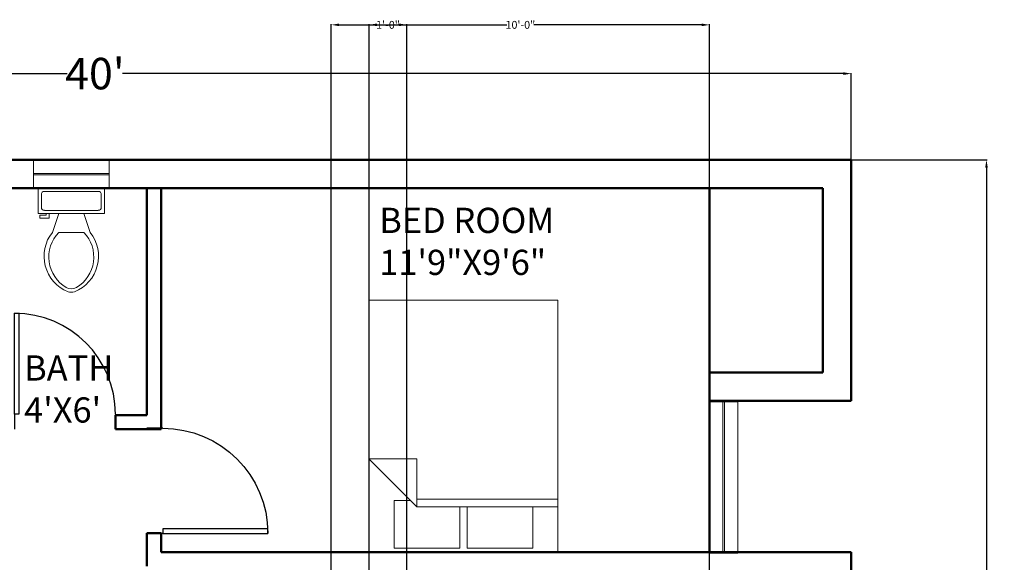
# Model space of a CAD drawing. Units: inches. Extents: x -46 to 565, y -56 to 809.
# Tile 6 of 6: x 252 to 565, y 636 to 809. Entities that reach past the tile are written whole.
import ezdxf

# ---------------------------------------------------------------- set-up
doc = ezdxf.new("R2010")
doc.units = ezdxf.units.IN
doc.header["$MEASUREMENT"] = 0
for name, color, linetype, lineweight in [('A-ANNO-DIMS', 2, 'Continuous', 18), ('A-AREA-IDEN', 241, 'Continuous', 18), ('A-FLOR-FIXT', 131, 'Continuous', 18), ('A-FURN', 131, 'Continuous', 18), ('DOOR', 210, 'Continuous', 25), ('WALL', 10, 'Continuous', 50), ('WINDOW', 170, 'Continuous', 18)]:
    doc.layers.add(name, color=color, linetype=linetype, lineweight=lineweight)
doc.styles.get("Standard").update_dxf_attribs({"font": 'arial.ttf'})
doc.dimstyles.get("Standard").update_dxf_attribs({"dimtxt": 2.5, "dimasz": 2.5, "dimexe": 0.18, "dimexo": 0.0625, "dimgap": 0.09, "dimtad": 0, "dimtih": 1, "dimtoh": 1, "dimzin": 0, "dimdsep": 46, "dimlunit": 3, "dimtxsty": 'Standard', "dimcen": 0.09, "dimadec": 0, "dimazin": 0, "dimtfac": 1, "dimtofl": 0, "dimtmove": 0, "dimatfit": 3, "dimfxl": 1, "dimtolj": 1, "dimtzin": 0, "dimarcsym": 0})

# ---------------------------------------------------------------- blocks, each defined once
blk = doc.blocks.new('*U2')
for p, q in [((0, 0), (0, -6)), ((40, 0), (40, -6))]:
    blk.add_line(p, q)
blk.add_lwpolyline([(0, 0), (0, 40), (1.75, 40), (1.75, 0)], close=True)
blk.add_arc((0, 0), 40, 0, 90)
blk = doc.blocks.new('Bed - Queen')
for p, q in [((0, -80.00003), (0, 0)), ((0, 0), (59.99999, 0)), ((59.99999, 0), (59.99999, -80.00003)), ((7.99999, -1.2), (28.79998, -1.2)), ((7.99999, -14.4), (7.99999, -1.2)), ((28.79998, -1.2), (28.79998, -14.4)), ((31.19999, -1.2), (51.99999, -1.2)), ((31.19999, -14.4), (31.19999, -1.2)), ((51.99999, -1.2), (51.99999, -16.4)), ((0, -14.4), (44.8, -14.4)), ((59.99999, -29.6), (44.8, -14.4)), ((44.8, -14.4), (44.8, -29.6)), ((44.8, -16.8), (0, -16.8)), ((51.99999, -16.4), (46.79936, -16.4)), ((44.8, -29.6), (59.99999, -29.6)), ((59.99999, -80.00003), (0, -80.00003))]:
    blk.add_line(p, q)
blk = doc.blocks.new('Toilet - top')
for p, q in [((9.5, -6), (9.5, -2)), ((-10, -8.5), (-8, -8.5)), ((-10, -9.5), (-10, -8.5)), ((-8, -8.5), (-8, -8)), ((-7, -8), (-7, -9.5)), ((-4, -8), (-6, -14)), ((4, -8), (6, -14)), ((-7, -9.5), (-10, -9.5)), ((4, -14), (-4, -14))]:
    blk.add_line(p, q)
blk.add_lwpolyline([(10.5, -8), (10.5, 0), (-10.5, 0), (-10.5, -8)], close=True)
for points in [[(-9.5, -2), (-9.5, -6)], [(8.5, -1), (-8.5, -1)], [(-8.5, -7), (8.5, -7)]]:
    blk.add_lwpolyline(points)
for centre, radius, start, end in [((-8.62, -1.88), 0.884, 81.8699, 188.1301), ((8.62, -1.88), 0.884, 351.8699, 98.1301), ((-8.62, -6.12), 0.884, 171.8699, 278.1301), ((8.62, -6.12), 0.884, 261.8699, 8.1301), ((3.52, -21.58), 12.17, 141.4691, 247.9714), ((4.2, -21.82), 11.33, 136.3677, 238.9468), ((-3.52, -21.58), 12.17, 292.0284, 38.5307), ((-4.2, -21.82), 11.33, 301.053, 43.6321), ((0, -27.88), 4, 245.7318, 294.2682), ((0, -29), 4, 254.8605, 285.1395)]:
    blk.add_arc(centre, radius, start, end)
blk = doc.blocks.new('*D14')
at = {"layer": 'A-ANNO-DIMS', "color": 0, "lineweight": -2, "transparency": 16777216}
for p, q in [((36.14, 764.26), (36.14, 791.8)), ((38.64, 791.62), (267.37, 791.62)), ((513.64, 791.62), (284.92, 791.62)), ((516.14, 764.26), (516.14, 791.8))]:
    blk.add_line(p, q, dxfattribs=at)
at = {"layer": 'A-ANNO-DIMS', "color": 0, "transparency": 16777216}
for points in [[(38.64, 792.04), (38.64, 791.2), (36.14, 791.62)], [(513.64, 792.04), (513.64, 791.2), (516.14, 791.62)]]:
    blk.add_solid(points, dxfattribs=at)
at = {"layer": 'Defpoints', "color": 0, "transparency": 16777216}
for p in [(516.14, 791.62), (36.14, 764.2), (516.14, 764.2)]:
    blk.add_point(p, dxfattribs=at)
at = {"layer": 'A-ANNO-DIMS', "color": 0, "transparency": 16777216, "insert": (276.14, 791.62), "char_height": 10, "attachment_point": 5}
blk.add_mtext("\\A1;40'", dxfattribs=at)
blk = doc.blocks.new('WIN-48IN')
for p, q in [((0, 4.75), (48, 4.75)), ((0, 4.25), (48, 4.25))]:
    blk.add_line(p, q)
blk.add_lwpolyline([(0, 0), (48, 0), (48, 9), (0, 9)], close=True)
blk = doc.blocks.new('WIN-24IN')
for p, q in [((4.25, 24), (4.25, 0)), ((4.75, 24), (4.75, 0))]:
    blk.add_line(p, q)
blk.add_lwpolyline([(0, 24), (0, 0), (9, 0), (9, 24)], close=True)
blk = doc.blocks.new('*D39')
at = {"layer": 'A-ANNO-DIMS', "color": 0, "lineweight": -2, "transparency": 16777216}
for p, q in [((516.21, 764.2), (559.22, 764.2)), ((559.04, 761.7), (559.04, 610.07)), ((559.04, 455.7), (559.04, 607.33)), ((507.21, 453.2), (559.22, 453.2))]:
    blk.add_line(p, q, dxfattribs=at)
at = {"layer": 'A-ANNO-DIMS', "color": 0, "transparency": 16777216}
for points in [[(558.63, 761.7), (559.46, 761.7), (559.04, 764.2)], [(558.63, 455.7), (559.46, 455.7), (559.04, 453.2)]]:
    blk.add_solid(points, dxfattribs=at)
at = {"layer": 'Defpoints', "color": 0, "transparency": 16777216}
for p in [(516.14, 764.2), (507.14, 453.2), (559.04, 453.2)]:
    blk.add_point(p, dxfattribs=at)
at = {"layer": 'A-ANNO-DIMS', "color": 0, "transparency": 16777216, "insert": (559.04, 608.7), "char_height": 2.5, "attachment_point": 5}
blk.add_mtext('\\A1;25\'-11"', dxfattribs=at)
blk = doc.blocks.new('*D41')
at = {"layer": 'A-ANNO-DIMS', "color": 0, "lineweight": -2, "transparency": 16777216}
for p, q in [((351.14, 417.26), (351.14, 807.28)), ((353.64, 807.1), (406.88, 807.1)), ((468.64, 807.1), (415.41, 807.1)), ((471.14, 417.26), (471.14, 807.28))]:
    blk.add_line(p, q, dxfattribs=at)
at = {"layer": 'A-ANNO-DIMS', "color": 0, "transparency": 16777216}
for points in [[(353.64, 807.52), (353.64, 806.68), (351.14, 807.1)], [(468.64, 807.52), (468.64, 806.68), (471.14, 807.1)]]:
    blk.add_solid(points, dxfattribs=at)
at = {"layer": 'Defpoints', "color": 0, "transparency": 16777216}
for p in [(471.14, 807.1), (351.14, 417.2), (471.14, 417.2)]:
    blk.add_point(p, dxfattribs=at)
at = {"layer": 'A-ANNO-DIMS', "color": 0, "transparency": 16777216, "insert": (411.14, 807.1), "char_height": 2.5, "attachment_point": 5}
blk.add_mtext('\\A1;10\'-0"', dxfattribs=at)
blk = doc.blocks.new('*D45')
at = {"layer": 'A-ANNO-DIMS', "color": 0, "lineweight": -2, "transparency": 16777216}
for p, q in [((363.14, 453.26), (363.14, 807.28)), ((365.64, 807.1), (365.85, 807.1)), ((372.64, 807.1), (372.44, 807.1)), ((375.14, 453.26), (375.14, 807.28))]:
    blk.add_line(p, q, dxfattribs=at)
at = {"layer": 'A-ANNO-DIMS', "color": 0, "transparency": 16777216}
for points in [[(365.64, 807.52), (365.64, 806.68), (363.14, 807.1)], [(372.64, 807.52), (372.64, 806.68), (375.14, 807.1)]]:
    blk.add_solid(points, dxfattribs=at)
at = {"layer": 'Defpoints', "color": 0, "transparency": 16777216}
for p in [(375.14, 807.1), (363.14, 453.2), (375.14, 453.2)]:
    blk.add_point(p, dxfattribs=at)
at = {"layer": 'A-ANNO-DIMS', "color": 0, "transparency": 16777216, "insert": (369.14, 807.1), "char_height": 2.5, "attachment_point": 5}
blk.add_mtext('\\A1;1\'-0"', dxfattribs=at)

msp = doc.modelspace()

# ---------------------------------------------------------------- linework, layer by layer
at = {"layer": 'WALL'}
for p, q in [((516.143, 764.2), (36.143, 764.2)), ((516.143, 687.7), (516.143, 764.2)), ((292.643, 755.2), (244.643, 755.2)), ((507.143, 755.2), (292.643, 755.2)), ((292.643, 755.2), (292.643, 683.2)), ((297.143, 755.2), (297.143, 678.7)), ((471.143, 639.7), (471.143, 755.2)), ((507.143, 696.7), (507.143, 755.2)), ((507.143, 696.7), (471.143, 696.7)), ((516.143, 687.7), (471.143, 687.7)), ((292.643, 683.2), (282.643, 683.2)), ((282.643, 683.2), (282.643, 678.7)), ((292.643, 678.7), (282.643, 678.7)), ((292.643, 678.7), (297.143, 678.7)), ((292.643, 645.7), (297.143, 645.7)), ((292.643, 645.7), (292.643, 639.7)), ((297.143, 645.7), (297.143, 639.7)), ((292.643, 639.7), (292.643, 635.2)), ((438.143, 639.7), (297.143, 639.7)), ((516.143, 639.7), (438.143, 639.7)), ((516.143, 551.2), (516.143, 639.7))]:
    msp.add_line(p, q, dxfattribs=at)

# ---------------------------------------------------------------- block references
at = {"layer": 'A-FLOR-FIXT'}
msp.add_blockref('Toilet - top', (268.643, 755.2), dxfattribs=at)
at = {"layer": 'A-FURN', "rotation": 180}
msp.add_blockref('Bed - Queen', (423.081, 639.7), dxfattribs=at)
at = {"layer": 'DOOR', "xscale": 0.8, "yscale": 0.8, "zscale": 0.8}
msp.add_blockref('*U2', (250.643, 683.5), dxfattribs=at)
at = {"layer": 'DOOR', "xscale": -0.834169050489643, "yscale": 0.834169050489643, "zscale": 0.834169050489643, "rotation": 270}
msp.add_blockref('*U2', (297.648, 645.639), dxfattribs=at)
at = {"layer": 'WINDOW'}
for name, p, rotation in [('WIN-24IN', (256.643, 764.2), 270.0000000000005), ('WIN-48IN', (471.143, 687.351), 270.0000000000001)]:
    msp.add_blockref(name, p, dxfattribs=dict(at, rotation=rotation))

# ---------------------------------------------------------------- texts
at = {"layer": 'A-AREA-IDEN', "char_height": 8, "attachment_point": 1}
for s, insert in [('BED ROOM\\P11\'9"X9\'6" ', (366.356, 749.015)), ("BATH\\P4'X6'", (253.676, 702.146))]:
    msp.add_mtext_dynamic_manual_height_columns(s, width=70.77133, gutter_width=1, heights=[0], dxfattribs=dict(at, insert=insert))

# ---------------------------------------------------------------- dimensions: what is measured, and where the dimension line sits
at = {"layer": 'A-ANNO-DIMS'}
for base, p1, p2, picture, middle in [((471.143, 807.1), (351.143, 417.2), (471.143, 417.2), '*D41', (411.143, 807.1)), ((375.143, 807.1), (363.143, 453.2), (375.143, 453.2), '*D45', (369.143, 807.1))]:
    dim = msp.add_linear_dim(base=base, p1=p1, p2=p2, dimstyle='Standard', override={"dimdec": 1, "dimlfac": 1, "dimrnd": 0, "dimzin": 1, "dimdsep": 46, "dimlunit": 4, "dimfrac": 2}, dxfattribs=at)
    dim.commit()
    dim.dimension.update_dxf_attribs({"geometry": picture, "text_midpoint": middle})
dim = msp.add_aligned_dim(p1=(36.143, 764.2), p2=(516.143, 764.2), distance=27.422, dimstyle='Standard', override={"dimtxt": 10, "dimclrd": 0, "dimclre": 0, "dimclrt": 0}, dxfattribs=at)
dim.commit()
dim.dimension.update_dxf_attribs({"geometry": '*D14', "text_midpoint": (276.143, 791.621)})
dim = msp.add_linear_dim(base=(559.043, 453.2), p1=(516.143, 764.2), p2=(507.143, 453.2), angle=90, dimstyle='Standard', override={"dimdec": 1, "dimlfac": 1, "dimrnd": 0, "dimzin": 1, "dimdsep": 46, "dimlunit": 4, "dimfrac": 2}, dxfattribs=at)
dim.commit()
dim.dimension.update_dxf_attribs({"geometry": '*D39', "text_midpoint": (559.043, 608.7)})

doc.saveas('drawing.dxf')
